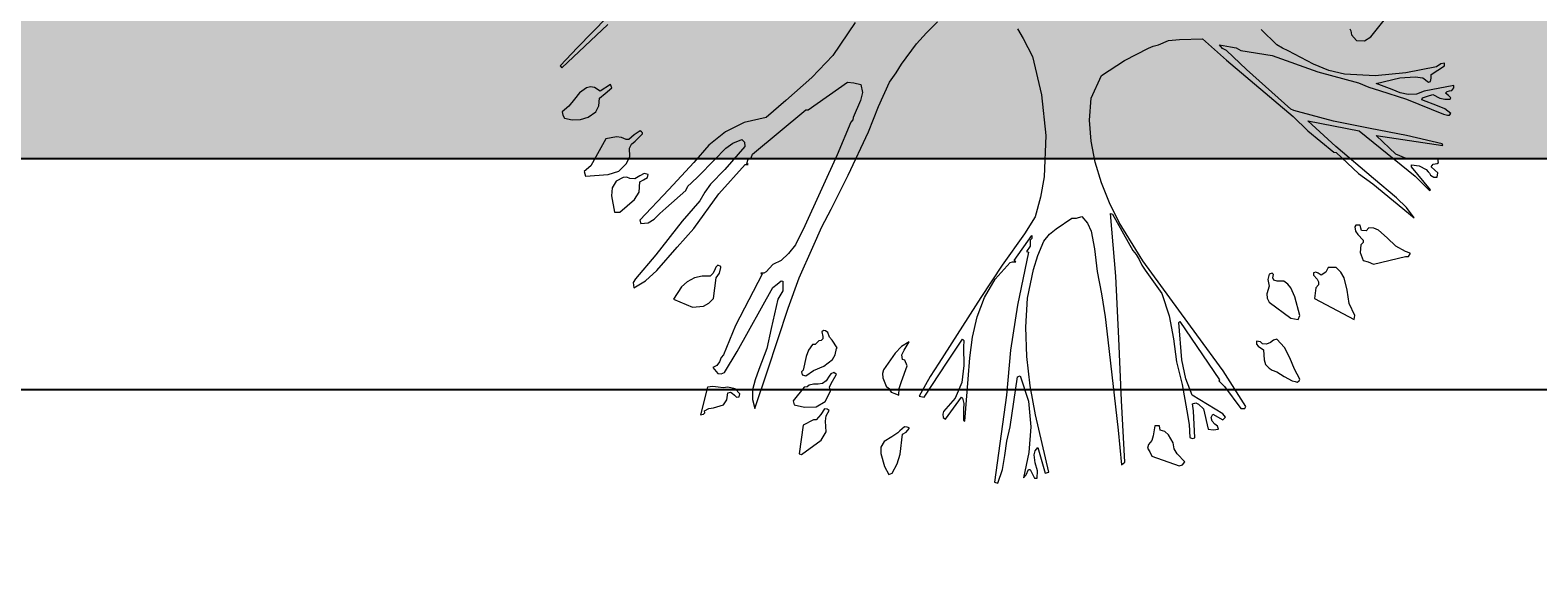
# Model space of a CAD drawing. Units: inches. Extents: x 84 to 1044, y -280 to 906.
# Tile 30 of 105: x 789 to 848, y -129 to -108. Entities that reach past the tile are written whole.
import ezdxf

# ---------------------------------------------------------------- set-up
doc = ezdxf.new("R2010")
doc.units = ezdxf.units.IN
for name, color, linetype, lineweight in [('A-ANNO-DIMS', 2, 'Continuous', 18), ('C-PROP', 7, 'Continuous', 25), ('L-PLNT', 114, 'Continuous', 15)]:
    doc.layers.add(name, color=color, linetype=linetype, lineweight=lineweight)
doc.layers.add('L-PLNT-PATT', color=9, linetype='Continuous', lineweight=9, true_color=0xafd9aa)
doc.styles.get("Standard").update_dxf_attribs({"font": 'arial.ttf'})
doc.dimstyles.get("Standard").update_dxf_attribs({"dimtxt": 0.18, "dimasz": 0.18, "dimexe": 0.18, "dimexo": 0.0625, "dimgap": 0.09, "dimtad": 0, "dimtih": 1, "dimtoh": 1, "dimdec": 4, "dimzin": 0, "dimdsep": 46, "dimtxsty": 'Standard', "dimcen": 0.09, "dimadec": 0, "dimazin": 0, "dimtfac": 1, "dimtdec": 4, "dimtofl": 0, "dimtmove": 0, "dimatfit": 3, "dimfxl": 1, "dimtolj": 1, "dimtzin": 0, "dimarcsym": 0})

# ---------------------------------------------------------------- blocks, each defined once
blk = doc.blocks.new('A$C37E508DF')
for p, q in [((1.3164, 0.7615), (1.3871, 0.6891)), ((0.1312, 0.7058), (0.1081, 0.7349)), ((0.1646, 0.7186), (0.1629, 0.7152)), ((0.28, 0.6933), (0.3049, 0.7178)), ((0.6903, 0.7186), (0.6818, 0.7032)), ((0.8344, 0.7122), (0.8173, 0.7298)), ((0.9476, 0.7285), (0.9828, 0.6762)), ((1.4116, 0.6569), (1.3391, 0.7255)), ((0.1415, 0.6994), (0.1312, 0.7058)), ((0.1539, 0.7002), (0.1415, 0.6994)), ((0.1621, 0.7092), (0.1539, 0.7002)), ((0.1629, 0.7152), (0.1621, 0.7092)), ((0.271, 0.6882), (0.28, 0.6933)), ((0.3709, 0.6933), (0.3533, 0.6903)), ((0.3975, 0.7028), (0.3598, 0.6693)), ((0.3662, 0.6873), (0.3709, 0.6933)), ((0.4339, 0.7019), (0.3975, 0.7028)), ((0.4515, 0.7002), (0.4339, 0.7019)), ((0.4674, 0.6933), (0.4515, 0.7002)), ((0.476, 0.6912), (0.4674, 0.6933)), ((0.6818, 0.7032), (0.6667, 0.6749)), ((0.8503, 0.6951), (0.8344, 0.7122)), ((0.8739, 0.6629), (0.8503, 0.6951)), ((0.2877, 0.6762), (0.2152, 0.6505)), ((0.2221, 0.6625), (0.262, 0.6839)), ((0.3598, 0.6693), (0.2543, 0.5797)), ((0.262, 0.6839), (0.271, 0.6882)), ((0.337, 0.6843), (0.2877, 0.6762)), ((0.328, 0.6543), (0.3598, 0.6843)), ((0.3443, 0.6886), (0.337, 0.6843)), ((0.3533, 0.6903), (0.3443, 0.6886)), ((0.3598, 0.6843), (0.3662, 0.6873)), ((0.4832, 0.6878), (0.476, 0.6912)), ((0.521, 0.6685), (0.4832, 0.6878)), ((0.5578, 0.6449), (0.521, 0.6685)), ((0.6667, 0.6749), (0.6526, 0.614)), ((0.9828, 0.6762), (1.0162, 0.6415)), ((1.3871, 0.6891), (1.4141, 0.6599)), ((0.0146, 0.6599), (0.0146, 0.6642)), ((0.0146, 0.6642), (0.0206, 0.6633)), ((0.036, 0.6466), (0.0146, 0.6599)), ((0.0206, 0.6633), (0.0274, 0.6586)), ((0.0274, 0.6586), (0.0759, 0.6492)), ((0.0356, 0.6406), (0.036, 0.6466)), ((0.0759, 0.6492), (0.1244, 0.644)), ((0.1244, 0.644), (0.1728, 0.647)), ((0.2152, 0.6505), (0.1509, 0.6333)), ((0.1728, 0.647), (0.1977, 0.6526)), ((0.1977, 0.6526), (0.2221, 0.6625)), ((0.2581, 0.5913), (0.328, 0.6543)), ((0.5737, 0.6089), (0.5578, 0.6449)), ((0.8824, 0.6492), (0.8739, 0.6629)), ((0.8932, 0.6342), (0.8824, 0.6492)), ((1.4141, 0.6599), (1.4116, 0.6569)), ((0, 0.629), (0.0467, 0.62)), ((0, 0.6252), (0, 0.629)), ((0.003, 0.6213), (0, 0.6252)), ((0.0069, 0.6204), (0.003, 0.6213)), ((0.0107, 0.6196), (0.0069, 0.6204)), ((0.0369, 0.6355), (0.0356, 0.6406)), ((0.0399, 0.6342), (0.0369, 0.6355)), ((0.0489, 0.641), (0.0399, 0.6342)), ((0.0609, 0.6428), (0.0489, 0.641)), ((0.0853, 0.641), (0.0609, 0.6428)), ((0.1175, 0.6213), (0.0746, 0.6076)), ((0.0849, 0.6175), (0.0973, 0.6226)), ((0.1226, 0.632), (0.0853, 0.641)), ((0.0973, 0.6226), (0.1226, 0.632)), ((0.1342, 0.6265), (0.1175, 0.6213)), ((0.1509, 0.6333), (0.1342, 0.6265)), ((0.9103, 0.5956), (0.8932, 0.6342)), ((0.9382, 0.6303), (0.936, 0.6179)), ((0.9493, 0.6333), (0.9382, 0.6303)), ((0.9596, 0.6342), (0.9493, 0.6333)), ((1.0218, 0.5904), (0.9596, 0.6342)), ((1.0162, 0.6415), (1.0574, 0.605)), ((1.3327, 0.6252), (1.3348, 0.6303)), ((1.343, 0.6162), (1.3327, 0.6252)), ((1.3348, 0.6303), (1.3511, 0.62)), ((1.3511, 0.62), (1.3601, 0.6256)), ((1.3601, 0.6256), (1.3661, 0.6269)), ((1.3661, 0.6269), (1.3725, 0.6252)), ((1.3725, 0.6252), (1.3837, 0.6175)), ((0.0047, 0.6093), (0.0086, 0.6132)), ((0.0056, 0.6076), (0.0047, 0.6093)), ((0.0141, 0.6072), (0.0056, 0.6076)), ((0.0086, 0.6132), (0.0133, 0.617)), ((0.0133, 0.617), (0.0107, 0.6196)), ((0.0223, 0.6089), (0.0141, 0.6072)), ((0.0141, 0.5921), (0.0257, 0.5969)), ((0.0746, 0.6076), (0.0163, 0.5836)), ((0.0334, 0.6145), (0.0223, 0.6089)), ((0.0257, 0.5969), (0.0506, 0.6063)), ((0.0416, 0.6119), (0.0334, 0.6145)), ((0.0493, 0.6093), (0.0416, 0.6119)), ((0.0467, 0.62), (0.0592, 0.6153)), ((0.0506, 0.6063), (0.0493, 0.6093)), ((0.0592, 0.6153), (0.072, 0.6149)), ((0.072, 0.6149), (0.0849, 0.6175)), ((0.5763, 0.5741), (0.5737, 0.6089)), ((0.6526, 0.614), (0.6457, 0.5497)), ((0.936, 0.6179), (0.939, 0.605)), ((0.939, 0.605), (0.9506, 0.5784)), ((1.0574, 0.605), (1.0883, 0.5784)), ((1.352, 0.6089), (1.343, 0.6162)), ((1.3533, 0.5969), (1.352, 0.6089)), ((1.358, 0.5874), (1.3533, 0.5969)), ((1.3837, 0.6175), (1.3918, 0.6072)), ((1.3918, 0.6072), (1.4004, 0.5964)), ((0.0047, 0.5849), (0.0141, 0.5921)), ((0.0069, 0.5823), (0.0047, 0.5849)), ((0.0099, 0.5823), (0.0069, 0.5823)), ((0.0163, 0.5836), (0.0099, 0.5823)), ((0.2311, 0.5729), (0.1496, 0.557)), ((0.1869, 0.5325), (0.2311, 0.5729)), ((0.1904, 0.5724), (0.2474, 0.5879)), ((0.2543, 0.5797), (0.2311, 0.557)), ((0.2474, 0.5879), (0.253, 0.5892)), ((0.253, 0.5892), (0.2581, 0.5913)), ((0.5737, 0.5407), (0.5763, 0.5741)), ((0.9262, 0.5557), (0.9103, 0.5956)), ((0.9506, 0.5784), (0.951, 0.5746)), ((0.951, 0.5746), (0.9545, 0.5711)), ((1.0256, 0.5904), (1.0218, 0.5904)), ((1.1097, 0.5205), (1.0256, 0.5904)), ((1.0883, 0.5784), (1.123, 0.5703)), ((1.37, 0.5789), (1.358, 0.5874)), ((1.3824, 0.575), (1.37, 0.5789)), ((1.3953, 0.5746), (1.3824, 0.575)), ((1.4077, 0.5771), (1.3953, 0.5746)), ((1.4004, 0.5964), (1.4111, 0.5874)), ((1.4103, 0.5823), (1.4077, 0.5771)), ((1.4111, 0.5874), (1.4103, 0.5823)), ((0.1226, 0.5497), (0.0171, 0.5338)), ((0.0184, 0.5368), (0.0746, 0.5501)), ((0.1496, 0.557), (0.0613, 0.4858)), ((0.0746, 0.5501), (0.1325, 0.5608)), ((0.0917, 0.5205), (0.1226, 0.5497)), ((0.1325, 0.5608), (0.1904, 0.5724)), ((0.2311, 0.557), (0.1899, 0.5235)), ((0.6457, 0.5497), (0.6483, 0.4845)), ((0.9583, 0.4871), (0.9262, 0.5557)), ((0.9545, 0.5711), (0.9759, 0.5193)), ((1.123, 0.5703), (1.1526, 0.5557)), ((1.1526, 0.5557), (1.1792, 0.5347)), ((1.2842, 0.554), (1.2855, 0.5557)), ((1.2842, 0.5527), (1.2842, 0.554)), ((1.2958, 0.5407), (1.2842, 0.5527)), ((1.2855, 0.5557), (1.2876, 0.557)), ((1.2876, 0.557), (1.2971, 0.551)), ((1.2971, 0.551), (1.3057, 0.5433)), ((0.0171, 0.5338), (0.0184, 0.5368)), ((0.1269, 0.482), (0.1869, 0.5325)), ((0.5677, 0.5077), (0.5737, 0.5407)), ((1.1226, 0.5394), (1.1221, 0.5325)), ((1.1221, 0.5325), (1.1539, 0.4961)), ((1.1268, 0.5433), (1.1226, 0.5394)), ((1.141, 0.5377), (1.1268, 0.5433)), ((1.1521, 0.5296), (1.141, 0.5377)), ((1.1706, 0.5111), (1.1521, 0.5296)), ((1.1792, 0.5347), (1.2027, 0.5072)), ((1.3014, 0.536), (1.2958, 0.5407)), ((1.3044, 0.53), (1.3014, 0.536)), ((1.3039, 0.5167), (1.3044, 0.53)), ((1.3057, 0.5433), (1.3099, 0.5433)), ((1.3099, 0.5433), (1.3172, 0.5467)), ((1.3172, 0.5467), (1.3254, 0.548)), ((1.3254, 0.548), (1.3421, 0.5446)), ((1.3421, 0.5446), (1.3657, 0.5021)), ((0.024, 0.5072), (0.0253, 0.5128)), ((0.0262, 0.5055), (0.024, 0.5072)), ((0.0253, 0.5128), (0.042, 0.5133)), ((0.0326, 0.5047), (0.0262, 0.5055)), ((0.036, 0.5004), (0.0326, 0.5047)), ((0.042, 0.5133), (0.0587, 0.5124)), ((0.0549, 0.5021), (0.0437, 0.4961)), ((0.0669, 0.5034), (0.0549, 0.5021)), ((0.0587, 0.5124), (0.0755, 0.5133)), ((0.0669, 0.5004), (0.0669, 0.5034)), ((0.0755, 0.5133), (0.0917, 0.5205)), ((0.1861, 0.5231), (0.1509, 0.4897)), ((0.1899, 0.5235), (0.1861, 0.5231)), ((0.5578, 0.4751), (0.5677, 0.5077)), ((0.9759, 0.5193), (1.0269, 0.4069)), ((1.1118, 0.5145), (1.1097, 0.5205)), ((1.117, 0.5124), (1.1118, 0.5145)), ((1.1191, 0.5055), (1.117, 0.5124)), ((1.117, 0.5042), (1.1191, 0.5055)), ((1.1217, 0.5042), (1.117, 0.5042)), ((1.1633, 0.4575), (1.1217, 0.5042)), ((1.1955, 0.4858), (1.1706, 0.5111)), ((1.2027, 0.5072), (1.2426, 0.4644)), ((1.3091, 0.5055), (1.3039, 0.5167)), ((1.3215, 0.4935), (1.3091, 0.5055)), ((1.3657, 0.5021), (1.3764, 0.4927)), ((0.0253, 0.491), (0.03, 0.4948)), ((0.0262, 0.4841), (0.0253, 0.491)), ((0.0317, 0.4841), (0.0262, 0.4841)), ((0.03, 0.4948), (0.036, 0.5004)), ((0.0369, 0.4871), (0.0317, 0.4841)), ((0.0369, 0.4639), (0.0669, 0.5004)), ((0.0382, 0.4905), (0.0369, 0.4871)), ((0.0403, 0.4922), (0.0382, 0.4905)), ((0.0613, 0.4858), (0.0386, 0.4627)), ((0.0437, 0.4961), (0.0403, 0.4922)), ((0.0905, 0.4515), (0.1269, 0.482)), ((0.1509, 0.4897), (0.1282, 0.4734)), ((0.6483, 0.4845), (0.6539, 0.4524)), ((0.9853, 0.4335), (0.9583, 0.4871)), ((1.1539, 0.4961), (1.1762, 0.4729)), ((1.207, 0.4747), (1.1955, 0.4858)), ((1.2748, 0.4884), (1.2812, 0.4897)), ((1.2761, 0.4832), (1.2748, 0.4884)), ((1.2825, 0.4798), (1.2761, 0.4832)), ((1.2812, 0.4897), (1.2885, 0.4862)), ((1.2885, 0.4764), (1.2825, 0.4798)), ((1.2885, 0.4862), (1.2962, 0.4815)), ((1.2962, 0.4815), (1.3039, 0.482)), ((1.3039, 0.482), (1.3087, 0.4841)), ((1.3087, 0.4841), (1.3147, 0.4832)), ((1.3147, 0.4832), (1.3258, 0.4777)), ((1.3382, 0.4884), (1.3215, 0.4935)), ((1.3258, 0.4777), (1.3318, 0.4669)), ((1.3743, 0.4858), (1.3382, 0.4884)), ((1.3764, 0.4927), (1.3743, 0.4858)), ((0.0386, 0.4627), (0.0369, 0.4639)), ((0.1282, 0.4734), (0.0626, 0.4198)), ((0.545, 0.4434), (0.5578, 0.4751)), ((1.2027, 0.4026), (1.1633, 0.4575)), ((1.1762, 0.4729), (1.1856, 0.4605)), ((1.1856, 0.4605), (1.1933, 0.4468)), ((1.2122, 0.47), (1.207, 0.4747)), ((1.2156, 0.4627), (1.2122, 0.47)), ((1.2469, 0.4348), (1.2156, 0.4627)), ((1.2426, 0.4644), (1.2885, 0.4159)), ((1.2894, 0.4601), (1.2885, 0.4764)), ((1.2967, 0.4485), (1.2894, 0.4601)), ((1.3331, 0.4545), (1.3284, 0.4284)), ((1.3318, 0.4669), (1.3331, 0.4545)), ((0.0626, 0.4198), (0.0746, 0.4361)), ((0.0746, 0.4361), (0.0905, 0.4515)), ((0.5295, 0.4125), (0.545, 0.4434)), ((0.6539, 0.4524), (0.6625, 0.4211)), ((1.0003, 0.4052), (0.9853, 0.4335)), ((1.1933, 0.4468), (1.2212, 0.4146)), ((1.2568, 0.4266), (1.2469, 0.4348)), ((1.3082, 0.4386), (1.2967, 0.4485)), ((1.3198, 0.4284), (1.3082, 0.4386)), ((0.1471, 0.4035), (0.1484, 0.4082)), ((0.1484, 0.4082), (0.1548, 0.4082)), ((0.1548, 0.4082), (0.1565, 0.4052)), ((0.4922, 0.3516), (0.5295, 0.4125)), ((0.5403, 0.4254), (0.5081, 0.3679)), ((0.5347, 0.3276), (0.5433, 0.4266)), ((0.5433, 0.4266), (0.5403, 0.4254)), ((0.5797, 0.4112), (0.5741, 0.3983)), ((0.5887, 0.4215), (0.5797, 0.4112)), ((0.5969, 0.4189), (0.5887, 0.4215)), ((0.6046, 0.4189), (0.5969, 0.4189)), ((0.6295, 0.4022), (0.6046, 0.4189)), ((0.6625, 0.4211), (0.6796, 0.3945)), ((1.0269, 0.4069), (1.0419, 0.3769)), ((1.2212, 0.4146), (1.2628, 0.361)), ((1.2658, 0.4176), (1.2568, 0.4266)), ((1.2752, 0.4116), (1.2658, 0.4176)), ((1.2868, 0.4108), (1.2752, 0.4116)), ((1.2885, 0.4159), (1.2868, 0.4108)), ((1.3284, 0.4284), (1.3198, 0.4284)), ((0.0917, 0.3748), (0.1055, 0.388)), ((0.1055, 0.388), (0.1192, 0.4001)), ((0.1192, 0.4001), (0.1265, 0.4031)), ((0.1265, 0.4031), (0.1346, 0.4039)), ((0.1346, 0.4039), (0.1389, 0.3992)), ((0.1389, 0.3992), (0.1458, 0.3996)), ((0.1518, 0.3932), (0.1432, 0.3842)), ((0.1432, 0.3842), (0.1436, 0.3808)), ((0.1458, 0.3996), (0.1471, 0.4035)), ((0.1556, 0.3983), (0.1518, 0.3932)), ((0.1565, 0.4052), (0.1556, 0.3983)), ((0.5741, 0.3983), (0.5686, 0.3705)), ((0.6397, 0.3936), (0.6295, 0.4022)), ((0.6487, 0.3825), (0.6397, 0.3936)), ((0.6582, 0.3602), (0.6487, 0.3825)), ((0.6959, 0.352), (0.668, 0.3919)), ((0.668, 0.3919), (0.668, 0.3872)), ((0.668, 0.3872), (0.6706, 0.3842)), ((0.6706, 0.3842), (0.6702, 0.3748)), ((0.6796, 0.3945), (0.7148, 0.3447)), ((1.0145, 0.373), (1.0003, 0.4052)), ((1.2289, 0.373), (1.2027, 0.4026)), ((0.069, 0.364), (0.0763, 0.3662)), ((0.069, 0.3627), (0.069, 0.364)), ((0.0716, 0.3585), (0.069, 0.3627)), ((0.0763, 0.3585), (0.0716, 0.3585)), ((0.0763, 0.3662), (0.0917, 0.3748)), ((0.1269, 0.3464), (0.0763, 0.3585)), ((0.1484, 0.3649), (0.1432, 0.352)), ((0.1436, 0.3808), (0.1471, 0.3769)), ((0.1471, 0.3769), (0.1484, 0.3649)), ((0.5025, 0.3619), (0.4982, 0.3537)), ((0.5081, 0.3679), (0.5025, 0.3619)), ((0.5686, 0.3705), (0.5643, 0.3349)), ((0.665, 0.3379), (0.6582, 0.3602)), ((0.6702, 0.3748), (0.6762, 0.3662)), ((0.6762, 0.3662), (0.6732, 0.3653)), ((0.6732, 0.3653), (0.6903, 0.2813)), ((1.0359, 0.3246), (1.0145, 0.373)), ((1.0419, 0.3769), (1.0527, 0.3632)), ((1.0527, 0.3632), (1.0647, 0.352)), ((1.2615, 0.3362), (1.2289, 0.373)), ((1.2628, 0.361), (1.2949, 0.3233)), ((0.1355, 0.3499), (0.1269, 0.3464)), ((0.1432, 0.352), (0.1355, 0.3499)), ((0.1788, 0.3336), (0.1861, 0.3409)), ((0.1861, 0.3409), (0.199, 0.3409)), ((0.199, 0.3409), (0.2024, 0.3336)), ((0.4065, 0.2345), (0.4922, 0.3516)), ((0.4884, 0.337), (0.4622, 0.2997)), ((0.4939, 0.3447), (0.4884, 0.337)), ((0.4982, 0.3537), (0.4939, 0.3447)), ((0.5643, 0.3349), (0.5578, 0.2993)), ((0.6745, 0.2924), (0.665, 0.3379)), ((0.6933, 0.3503), (0.6959, 0.352)), ((0.6985, 0.3503), (0.6933, 0.3503)), ((0.7023, 0.349), (0.6985, 0.3503)), ((0.7259, 0.3224), (0.7023, 0.349)), ((0.7148, 0.3447), (0.7487, 0.2937)), ((1.0647, 0.352), (1.078, 0.346)), ((1.078, 0.346), (1.0883, 0.334)), ((1.1599, 0.3426), (1.1646, 0.3447)), ((1.1599, 0.3413), (1.1599, 0.3426)), ((1.162, 0.3319), (1.1599, 0.3413)), ((1.1646, 0.3447), (1.168, 0.3417)), ((1.168, 0.3417), (1.1702, 0.3366)), ((1.1702, 0.3366), (1.1727, 0.3314)), ((1.2795, 0.3199), (1.2615, 0.3362)), ((0.1689, 0.3053), (0.1737, 0.325)), ((0.1737, 0.325), (0.1788, 0.3336)), ((0.2024, 0.3336), (0.2097, 0.3289)), ((0.2097, 0.3289), (0.2148, 0.3323)), ((0.2161, 0.3224), (0.214, 0.3186)), ((0.214, 0.3186), (0.214, 0.3139)), ((0.214, 0.3139), (0.2182, 0.3087)), ((0.2148, 0.3323), (0.2182, 0.3336)), ((0.2221, 0.3289), (0.2161, 0.3224)), ((0.2182, 0.3336), (0.2221, 0.3327)), ((0.2221, 0.3327), (0.2221, 0.3289)), ((0.2577, 0.3087), (0.2624, 0.3147)), ((0.2624, 0.3147), (0.2689, 0.3194)), ((0.2689, 0.3194), (0.2796, 0.3194)), ((0.2796, 0.3194), (0.2847, 0.3211)), ((0.2847, 0.3211), (0.2864, 0.325)), ((0.2851, 0.3302), (0.2877, 0.3319)), ((0.2864, 0.325), (0.2851, 0.3302)), ((0.2877, 0.3319), (0.292, 0.3306)), ((0.292, 0.3306), (0.2941, 0.322)), ((0.2941, 0.322), (0.292, 0.3117)), ((0.292, 0.3117), (0.2959, 0.2993)), ((0.53, 0.229), (0.5347, 0.3276)), ((0.7427, 0.2937), (0.7259, 0.3224)), ((1.0535, 0.2766), (1.0359, 0.3246)), ((1.0647, 0.3199), (1.0617, 0.3194)), ((1.0617, 0.3194), (1.0617, 0.304)), ((1.0711, 0.3147), (1.0647, 0.3199)), ((1.0775, 0.3092), (1.0711, 0.3147)), ((1.0883, 0.334), (1.0921, 0.3319)), ((1.0921, 0.3319), (1.0968, 0.3319)), ((1.0968, 0.3319), (1.0947, 0.3306)), ((1.0947, 0.3306), (1.1367, 0.2491)), ((1.1676, 0.325), (1.162, 0.3319)), ((1.1719, 0.292), (1.1676, 0.325)), ((1.1727, 0.3314), (1.177, 0.3276)), ((1.177, 0.3276), (1.1895, 0.3276)), ((1.1895, 0.3276), (1.2019, 0.3246)), ((1.2019, 0.3246), (1.2135, 0.3186)), ((1.2135, 0.3186), (1.2225, 0.3104)), ((1.2225, 0.3104), (1.2349, 0.2911)), ((1.2975, 0.3087), (1.2795, 0.3199)), ((1.2949, 0.3233), (1.2988, 0.3173)), ((1.2988, 0.3173), (1.2975, 0.3087)), ((0.2204, 0.292), (0.1578, 0.259)), ((0.1655, 0.2843), (0.1689, 0.3053)), ((0.2182, 0.3087), (0.2204, 0.292)), ((0.2436, 0.265), (0.2517, 0.2946)), ((0.2517, 0.2946), (0.2577, 0.3087)), ((0.2954, 0.2928), (0.292, 0.286)), ((0.2959, 0.2993), (0.2954, 0.2928)), ((0.4622, 0.2997), (0.4502, 0.2645)), ((0.5578, 0.2993), (0.5518, 0.2633)), ((0.6775, 0.2465), (0.6745, 0.2924)), ((0.7542, 0.2628), (0.7427, 0.2937)), ((0.7487, 0.2937), (0.8151, 0.1899)), ((1.0617, 0.304), (1.0698, 0.2911)), ((1.0698, 0.2911), (1.0805, 0.2448)), ((1.1341, 0.2084), (1.0775, 0.3092)), ((1.1792, 0.2847), (1.1719, 0.292)), ((1.2349, 0.2911), (1.2049, 0.2783)), ((0.1565, 0.265), (0.1655, 0.2843)), ((0.1578, 0.259), (0.1565, 0.265)), ((0.2461, 0.259), (0.2436, 0.265)), ((0.292, 0.286), (0.2581, 0.2607)), ((0.4502, 0.2645), (0.4438, 0.2285)), ((0.5518, 0.2633), (0.5475, 0.2268)), ((0.6903, 0.2813), (0.7015, 0.2101)), ((0.7615, 0.2311), (0.7542, 0.2628)), ((1.0861, 0.1775), (1.0535, 0.2766)), ((1.1873, 0.28), (1.1792, 0.2847)), ((1.2049, 0.2783), (1.1873, 0.28)), ((0.2581, 0.2607), (0.2461, 0.259)), ((0.4335, 0.2556), (0.3709, 0.1634)), ((0.4305, 0.1951), (0.4352, 0.2543)), ((0.4352, 0.2543), (0.4335, 0.2556)), ((0.6758, 0.2002), (0.6775, 0.2465)), ((0.9905, 0.2384), (0.9943, 0.241)), ((0.9943, 0.241), (0.9973, 0.2414)), ((0.9973, 0.2414), (1.0003, 0.2393)), ((1.0003, 0.2393), (0.9986, 0.232)), ((1.0805, 0.2448), (1.087, 0.2127)), ((1.1367, 0.2491), (1.1556, 0.2032)), ((0.2594, 0.1981), (0.268, 0.2148)), ((0.268, 0.2148), (0.28, 0.2277)), ((0.28, 0.2277), (0.2851, 0.226)), ((0.2851, 0.226), (0.2903, 0.2225)), ((0.2903, 0.2225), (0.2963, 0.22)), ((0.2963, 0.22), (0.3027, 0.2204)), ((0.3096, 0.2165), (0.301, 0.211)), ((0.3027, 0.2204), (0.3061, 0.2234)), ((0.3061, 0.2234), (0.3122, 0.2247)), ((0.3122, 0.22), (0.3096, 0.2165)), ((0.3122, 0.2247), (0.3122, 0.22)), ((0.3649, 0.1775), (0.4065, 0.2345)), ((0.4438, 0.2285), (0.4391, 0.1921)), ((0.5261, 0.1308), (0.53, 0.229)), ((0.5475, 0.2268), (0.5313, 0.084)), ((0.7662, 0.1981), (0.7615, 0.2311)), ((0.7778, 0.2277), (0.7752, 0.2255)), ((0.7752, 0.2255), (0.7761, 0.2152)), ((0.7761, 0.2152), (0.7752, 0.1861)), ((0.8018, 0.1912), (0.7778, 0.2277)), ((0.8619, 0.2234), (0.8739, 0.2161)), ((0.87, 0.2101), (0.8619, 0.2234)), ((0.8739, 0.2161), (0.8841, 0.2054)), ((0.9759, 0.214), (0.9836, 0.226)), ((0.9836, 0.226), (0.9879, 0.2311)), ((0.9879, 0.2311), (0.9905, 0.2384)), ((0.9986, 0.232), (0.9986, 0.2281)), ((0.9986, 0.2281), (1.0012, 0.2255)), ((1.0012, 0.2255), (1.0051, 0.2251)), ((1.0051, 0.2251), (1.0076, 0.2225)), ((1.0076, 0.2225), (1.0106, 0.2195)), ((1.0106, 0.2195), (1.0149, 0.2191)), ((1.0149, 0.2191), (1.0214, 0.2101)), ((0.2521, 0.1805), (0.2594, 0.1981)), ((0.3002, 0.1951), (0.298, 0.1874)), ((0.301, 0.211), (0.3002, 0.1951)), ((0.4241, 0.1651), (0.4305, 0.1951)), ((0.4391, 0.1921), (0.4301, 0.1561)), ((0.6706, 0.1539), (0.6758, 0.2002)), ((0.7015, 0.2101), (0.7079, 0.1389)), ((0.7688, 0.1646), (0.7662, 0.1981)), ((0.8383, 0.1359), (0.8018, 0.1912)), ((0.8649, 0.1857), (0.8687, 0.1947)), ((0.8687, 0.1947), (0.8726, 0.1955)), ((0.8734, 0.2032), (0.87, 0.2101)), ((0.8726, 0.1955), (0.8734, 0.2032)), ((0.8841, 0.2054), (0.9026, 0.1792)), ((0.9768, 0.2127), (0.9759, 0.214)), ((0.9789, 0.2028), (0.9768, 0.2127)), ((0.9832, 0.1955), (0.9789, 0.2028)), ((0.9969, 0.1852), (0.9832, 0.1955)), ((1.0214, 0.2101), (1.0252, 0.2002)), ((1.0252, 0.2002), (1.0295, 0.1788)), ((1.087, 0.2127), (1.0998, 0.1797)), ((1.1543, 0.1749), (1.1341, 0.2084)), ((1.1556, 0.2032), (1.1594, 0.1985)), ((1.1594, 0.1985), (1.1624, 0.1921)), ((1.1624, 0.1921), (1.1663, 0.1861)), ((0.2436, 0.1642), (0.2521, 0.1805)), ((0.2684, 0.1689), (0.2556, 0.1616)), ((0.28, 0.1762), (0.2684, 0.1689)), ((0.2873, 0.1788), (0.28, 0.1762)), ((0.292, 0.1818), (0.2873, 0.1788)), ((0.298, 0.1874), (0.292, 0.1818)), ((0.3293, 0.1213), (0.3649, 0.1775)), ((0.6865, 0.1698), (0.6732, 0.1295)), ((0.6903, 0.1681), (0.6865, 0.1698)), ((0.7023, 0.0892), (0.6903, 0.1681)), ((0.7752, 0.1861), (0.7787, 0.1591)), ((0.8151, 0.1899), (0.8288, 0.1685)), ((0.8288, 0.1685), (0.846, 0.1376)), ((0.8743, 0.1608), (0.8649, 0.1857)), ((0.9026, 0.1792), (0.9043, 0.1732)), ((0.9043, 0.1732), (0.9035, 0.1668)), ((0.9768, 0.1719), (0.9811, 0.1749)), ((0.9776, 0.1711), (0.9768, 0.1719)), ((0.9853, 0.1578), (0.9776, 0.1711)), ((0.9811, 0.1749), (0.9858, 0.1728)), ((0.9858, 0.1728), (0.9884, 0.1694)), ((0.9884, 0.1694), (0.9931, 0.1616)), ((1.0132, 0.1779), (0.9969, 0.1852)), ((1.0256, 0.1698), (1.0132, 0.1779)), ((1.0312, 0.1711), (1.0256, 0.1698)), ((1.0295, 0.1788), (1.0325, 0.1762)), ((1.0325, 0.1762), (1.0312, 0.1711)), ((1.1063, 0.1183), (1.0861, 0.1775)), ((1.0998, 0.1797), (1.1058, 0.1634)), ((1.1594, 0.1728), (1.1543, 0.1749)), ((1.1646, 0.1732), (1.1594, 0.1728)), ((1.1727, 0.1827), (1.1646, 0.1732)), ((1.1663, 0.1861), (1.1727, 0.1827)), ((0.2448, 0.1616), (0.2436, 0.1642)), ((0.2478, 0.1599), (0.2448, 0.1616)), ((0.2508, 0.1608), (0.2478, 0.1599)), ((0.2556, 0.1616), (0.2508, 0.1608)), ((0.3628, 0.1526), (0.337, 0.1183)), ((0.3692, 0.1591), (0.3628, 0.1526)), ((0.3718, 0.1616), (0.3692, 0.1591)), ((0.3709, 0.1634), (0.3718, 0.1616)), ((0.4138, 0.1389), (0.4241, 0.1651)), ((0.4301, 0.1561), (0.4224, 0.1145)), ((0.662, 0.108), (0.6706, 0.1539)), ((0.774, 0.0982), (0.7688, 0.1646)), ((0.7787, 0.1591), (0.789, 0.1346)), ((0.8777, 0.1496), (0.8743, 0.1608)), ((0.8781, 0.1389), (0.8777, 0.1496)), ((0.8902, 0.1441), (0.8846, 0.1419)), ((0.894, 0.1496), (0.8902, 0.1441)), ((0.8983, 0.1535), (0.894, 0.1496)), ((0.9035, 0.1668), (0.8983, 0.1535)), ((0.9879, 0.1518), (0.9853, 0.1578)), ((0.9866, 0.1453), (0.9879, 0.1518)), ((0.9948, 0.1291), (0.9866, 0.1453)), ((0.9931, 0.1616), (0.9991, 0.1574)), ((0.9991, 0.1574), (1.0059, 0.1565)), ((1.0059, 0.1565), (1.0132, 0.1565)), ((1.0132, 0.1565), (1.0205, 0.1548)), ((1.0205, 0.1548), (1.0235, 0.1522)), ((1.0235, 0.1522), (1.0282, 0.1518)), ((1.0282, 0.1518), (1.0454, 0.1303)), ((1.1058, 0.1634), (1.1097, 0.1475)), ((1.1097, 0.1475), (1.1101, 0.1325)), ((1.1298, 0.1411), (1.1376, 0.1492)), ((1.1376, 0.1492), (1.1491, 0.1518)), ((1.1449, 0.1441), (1.1423, 0.1423)), ((1.1491, 0.1428), (1.1449, 0.1441)), ((1.1491, 0.1518), (1.1564, 0.1505)), ((1.1564, 0.1505), (1.1642, 0.1518)), ((1.1642, 0.1518), (1.1727, 0.1531)), ((1.1727, 0.1531), (1.1813, 0.1518)), ((1.1813, 0.1518), (1.192, 0.108)), ((0.3306, 0.1183), (0.3293, 0.1213)), ((0.3653, 0.1098), (0.4138, 0.1389)), ((0.4039, 0.1248), (0.3962, 0.1175)), ((0.4082, 0.1269), (0.4039, 0.1248)), ((0.4134, 0.1256), (0.4082, 0.1269)), ((0.4121, 0.1145), (0.4134, 0.1256)), ((0.5205, 0.033), (0.5261, 0.1308)), ((0.6732, 0.1295), (0.6693, 0.0892)), ((0.7079, 0.1389), (0.7268, 0.0013)), ((0.7774, 0.1346), (0.7757, 0.1261)), ((0.7757, 0.1261), (0.7761, 0.117)), ((0.7791, 0.1359), (0.7774, 0.1346)), ((0.8044, 0.1012), (0.7791, 0.1359)), ((0.789, 0.1346), (0.8074, 0.1132)), ((0.846, 0.1376), (0.8383, 0.1359)), ((0.8846, 0.1419), (0.8781, 0.1389)), ((1.0089, 0.1205), (0.9948, 0.1291)), ((1.0274, 0.12), (1.0089, 0.1205)), ((1.0441, 0.1239), (1.0274, 0.12)), ((1.0454, 0.1303), (1.0441, 0.1239)), ((1.1101, 0.1325), (1.1063, 0.1183)), ((1.1311, 0.1364), (1.1298, 0.1411)), ((1.1354, 0.1359), (1.1311, 0.1364)), ((1.1384, 0.1389), (1.1354, 0.1359)), ((1.1423, 0.1423), (1.1384, 0.1389)), ((1.1504, 0.132), (1.1491, 0.1428)), ((1.1556, 0.1239), (1.1504, 0.132)), ((1.1714, 0.1192), (1.1556, 0.1239)), ((0.337, 0.1183), (0.3306, 0.1183)), ((0.3615, 0.1042), (0.3653, 0.1098)), ((0.3653, 0.0999), (0.3615, 0.1042)), ((0.3812, 0.1089), (0.3653, 0.0999)), ((0.3782, 0.0935), (0.3825, 0.0978)), ((0.3842, 0.1037), (0.3812, 0.1089)), ((0.3825, 0.0978), (0.3842, 0.1037)), ((0.3962, 0.1175), (0.3885, 0.0853)), ((0.4099, 0.0716), (0.4121, 0.1145)), ((0.4224, 0.1145), (0.4189, 0.093)), ((0.641, 0.0172), (0.662, 0.108)), ((0.7761, 0.099), (0.774, 0.0982)), ((0.7761, 0.117), (0.7761, 0.099)), ((0.8083, 0.1037), (0.8044, 0.1012)), ((0.8074, 0.1132), (0.8087, 0.1089)), ((0.8087, 0.1089), (0.8083, 0.1037)), ((0.9884, 0.1149), (0.9918, 0.117)), ((0.9935, 0.1063), (0.9884, 0.1149)), ((0.9918, 0.117), (0.9961, 0.1175)), ((0.9931, 0.081), (0.9943, 0.0982)), ((0.9943, 0.0982), (0.9935, 0.1063)), ((0.9961, 0.1175), (1.0016, 0.1085)), ((1.0016, 0.1085), (1.0089, 0.0999)), ((1.0089, 0.0999), (1.0132, 0.0999)), ((1.0132, 0.0999), (1.0295, 0.0917)), ((1.1792, 0.1179), (1.1714, 0.1192)), ((1.186, 0.1145), (1.1792, 0.1179)), ((1.1856, 0.111), (1.186, 0.1145)), ((1.1873, 0.1093), (1.1856, 0.111)), ((1.192, 0.108), (1.1873, 0.1093)), ((0.3722, 0.0853), (0.3739, 0.09)), ((0.3808, 0.0845), (0.3722, 0.0853)), ((0.3739, 0.09), (0.3782, 0.0935)), ((0.3885, 0.0853), (0.3808, 0.0845)), ((0.4142, 0.0707), (0.4099, 0.0716)), ((0.4176, 0.072), (0.4142, 0.0707)), ((0.4189, 0.093), (0.4176, 0.072)), ((0.4442, 0.0639), (0.4515, 0.0763)), ((0.4515, 0.0763), (0.4571, 0.0815)), ((0.4571, 0.0815), (0.4648, 0.084)), ((0.4648, 0.084), (0.4657, 0.0905)), ((0.4657, 0.0905), (0.473, 0.0905)), ((0.473, 0.0905), (0.476, 0.0746)), ((0.476, 0.0746), (0.4777, 0.0673)), ((0.5313, 0.084), (0.5257, 0.0291)), ((0.6693, 0.0892), (0.6728, 0.0484)), ((0.7075, 0.0665), (0.7023, 0.0892)), ((0.8619, 0.0875), (0.8649, 0.0887)), ((0.8619, 0.0866), (0.8619, 0.0875)), ((0.8666, 0.0806), (0.8619, 0.0866)), ((0.8649, 0.0887), (0.8691, 0.0892)), ((0.8726, 0.0776), (0.8666, 0.0806)), ((0.8691, 0.0892), (0.8769, 0.0827)), ((0.8764, 0.0459), (0.8726, 0.0776)), ((0.8769, 0.0827), (0.8799, 0.0797)), ((0.8799, 0.0797), (0.8893, 0.0733)), ((0.8893, 0.0733), (0.9013, 0.066)), ((1.0012, 0.0677), (0.9931, 0.081)), ((1.0295, 0.0917), (1.0359, 0.0463)), ((0.4378, 0.0463), (0.4425, 0.0544)), ((0.4425, 0.0544), (0.4442, 0.0639)), ((0.4777, 0.0673), (0.4832, 0.0613)), ((0.4811, 0.0493), (0.4777, 0.0424)), ((0.4845, 0.0553), (0.4811, 0.0493)), ((0.4832, 0.0613), (0.4845, 0.0553)), ((0.6582, 0.0562), (0.6466, 0.0159)), ((0.6625, 0.051), (0.6582, 0.0562)), ((0.6642, 0.045), (0.6625, 0.051)), ((0.6728, 0.0484), (0.6809, 0.0082)), ((0.7105, 0.0437), (0.7075, 0.0665)), ((0.9013, 0.066), (0.9069, 0.057)), ((0.9069, 0.057), (0.9069, 0.0471)), ((1.0325, 0.0454), (1.0012, 0.0677)), ((0.4258, 0.0339), (0.4378, 0.0463)), ((0.4296, 0.0291), (0.4258, 0.0339)), ((0.4348, 0.0274), (0.4296, 0.0291)), ((0.4777, 0.0424), (0.4348, 0.0274)), ((0.5257, 0.0291), (0.5205, 0.033)), ((0.659, 0.0193), (0.6625, 0.0321)), ((0.6625, 0.0321), (0.6642, 0.045)), ((0.7144, 0.0214), (0.7105, 0.0437)), ((0.8807, 0.0304), (0.8764, 0.0459)), ((0.8889, 0.0159), (0.8807, 0.0304)), ((0.9009, 0.0261), (0.894, 0.0137)), ((0.9069, 0.0471), (0.9009, 0.0261)), ((1.0359, 0.0463), (1.0325, 0.0454)), ((0.6466, 0.0159), (0.641, 0.0172)), ((0.6595, 0.0077), (0.659, 0.0193)), ((0.6637, 0.0077), (0.6595, 0.0077)), ((0.6702, 0.0214), (0.6637, 0.0077)), ((0.6732, 0.0214), (0.6702, 0.0214)), ((0.6766, 0.0133), (0.6732, 0.0214)), ((0.6809, 0.0082), (0.6766, 0.0133)), ((0.7216, 0), (0.7144, 0.0214)), ((0.7268, 0.0013), (0.7216, 0)), ((0.894, 0.0137), (0.8889, 0.0159))]:
    blk.add_line(p, q)
blk = doc.blocks.new('*D60')
at = {"layer": 'A-ANNO-DIMS', "color": 0, "lineweight": -2, "transparency": 16777216}
for p, q in [((134.179, -121.942), (134.179, -180.64)), ((992.074, -121.942), (992.074, -180.64)), ((134.359, -180.46), (562.733, -180.46)), ((991.894, -180.46), (563.521, -180.46))]:
    blk.add_line(p, q, dxfattribs=at)
at = {"layer": 'A-ANNO-DIMS', "color": 0, "transparency": 16777216}
for points in [[(134.359, -180.43), (134.359, -180.49), (134.179, -180.46)], [(991.894, -180.43), (991.894, -180.49), (992.074, -180.46)]]:
    blk.add_solid(points, dxfattribs=at)
at = {"layer": 'Defpoints', "color": 0, "transparency": 16777216}
for p in [(134.179, -121.88), (992.074, -121.88), (992.074, -180.46)]:
    blk.add_point(p, dxfattribs=at)
at = {"layer": 'A-ANNO-DIMS', "color": 0, "transparency": 16777216, "insert": (563.127, -180.46), "char_height": 0.18, "attachment_point": 5}
blk.add_mtext('\\A1;857.9', dxfattribs=at)

msp = doc.modelspace()

# ---------------------------------------------------------------- hatches: boundary and pattern name
at = {"layer": 'L-PLNT-PATT', "transparency": 33554597}
h = msp.add_hatch(color=256, dxfattribs=at)
h.dxf.hatch_style = 1
h.paths.add_polyline_path([(791.074, 31.12), (791.074, 91.12), (743.074, 91.12), (674.074, 91.12), (674.074, 31.12), (650.074, 31.12), (650.074, -112.88), (983.074, -112.88), (983.074, -64.88), (791.074, -64.88)])

# ---------------------------------------------------------------- linework, layer by layer
at = {"layer": 'C-PROP'}
for points in [[(143.179, -121.88), (134.179, -121.88), (134.179, 856.12), (992.074, 856.12), (992.074, -121.88), (624.574, -121.88)], [(143.179, -112.88), (143.179, 847.12), (983.074, 847.12), (983.074, -112.88), (624.574, -112.88)]]:
    msp.add_lwpolyline(points, dxfattribs=at)

# ---------------------------------------------------------------- block references
at = {"layer": 'L-PLNT', "xscale": -24.64361536662419, "yscale": 24.64361536662419, "zscale": 24.64361536662419}
msp.add_blockref('A$C37E508DF', (844.575, -125.52), dxfattribs=at)

# ---------------------------------------------------------------- dimensions: what is measured, and where the dimension line sits
at = {"layer": 'A-ANNO-DIMS'}
dim = msp.add_linear_dim(base=(992.074, -180.46), p1=(134.179, -121.88), p2=(992.074, -121.88), dimstyle='Standard', override={"dimdec": 1, "dimlfac": 1, "dimrnd": 0, "dimzin": 0, "dimdsep": 46, "dimlunit": 2}, dxfattribs=at)
dim.commit()
dim.dimension.update_dxf_attribs({"geometry": '*D60', "text_midpoint": (563.127, -180.46)})

doc.saveas('drawing.dxf')
